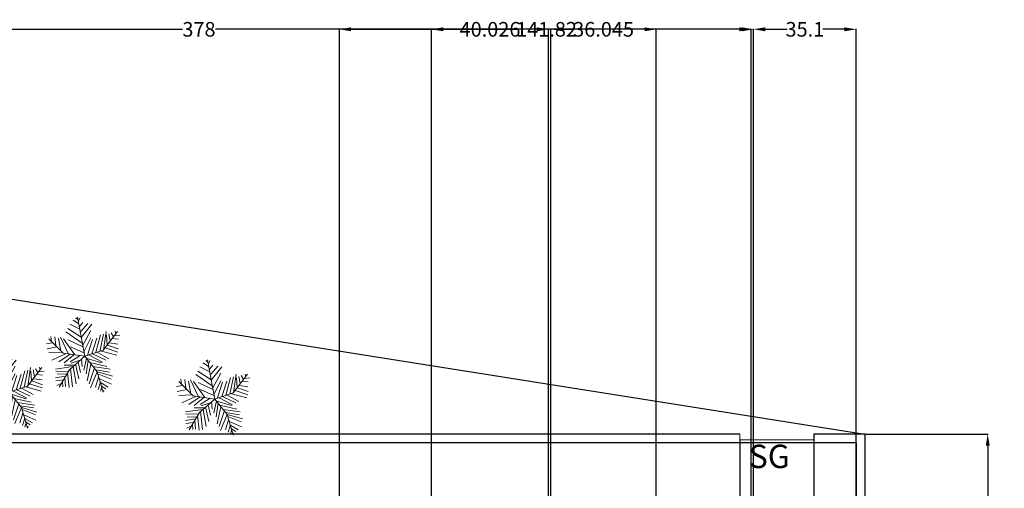
# Model space of a CAD drawing. Units: inches. Extents: x 460 to 1030, y -658 to 271.
# Tile 10 of 10: x 690 to 1028, y 111 to 271. Entities that reach past the tile are written whole.
import ezdxf

# ---------------------------------------------------------------- set-up
doc = ezdxf.new("R2010")
doc.units = ezdxf.units.IN
doc.header["$MEASUREMENT"] = 0
for name, color, linetype, lineweight in [('A-ANNO-DIMS', 2, 'Continuous', 18), ('A-ANNO-TEXT', 7, 'Continuous', 18), ('C-PROP', 7, 'Continuous', 25), ('C-SITE-GATE', 3, 'Continuous', 18), ('L-PLNT', 94, 'Continuous', 13)]:
    doc.layers.add(name, color=color, linetype=linetype, lineweight=lineweight)
doc.styles.get("Standard").update_dxf_attribs({"font": 'arial.ttf'})
doc.dimstyles.get("Standard").update_dxf_attribs({"dimtxt": 5, "dimasz": 4, "dimexe": 0.18, "dimexo": 0.0625, "dimgap": 0.09, "dimtad": 0, "dimtih": 1, "dimtoh": 1, "dimdec": 1, "dimzin": 0, "dimdsep": 46, "dimlunit": 4, "dimtxsty": 'Standard', "dimcen": 0.09, "dimadec": 0, "dimazin": 0, "dimtfac": 1, "dimtdec": 1, "dimtofl": 0, "dimtmove": 0, "dimatfit": 3, "dimfxl": 1, "dimtolj": 1, "dimtzin": 0, "dimarcsym": 0})

# ---------------------------------------------------------------- blocks, each defined once
blk = doc.blocks.new('*U11')
for p, q in [((-185.1152, 1008.5578), (-553.1612, 1185.4942)), ((-221.9198, 1197.3052), (-433.5526, 1338.8594)), ((-258.7244, 1362.456), (-332.3336, 1421.4348)), ((0, 0), (-266.7, 1447.8)), ((-231.1146, 1315.2628), (-166.7002, 1421.4348)), ((-194.31, 1102.9442), (-65.4812, 1256.284)), ((-148.3106, 914.1968), (118.5418, 1220.9018)), ((-129.8956, 701.8528), (265.7602, 1185.4942)), ((-1234.059, 536.7274), (-1252.4486, 737.2604)), ((-93.091, 489.5342), (-700.3796, 902.3858)), ((-129.8956, 713.6638), (-626.7704, 1032.1544)), ((-74.7014, 418.7444), (219.7608, 961.39)), ((412.9786, 147.447), (587.8068, 796.2392)), ((560.197, 182.8292), (698.2206, 819.8358)), ((685.8, 228.6), (1219.2, 914.4)), ((689.0258, 230.0224), (790.2448, 914.1968)), ((808.6344, 784.4282), (827.0494, 418.7444)), ((891.4384, 831.6214), (946.658, 572.1096)), ((983.4626, 867.0036), (1066.2666, 725.4494)), ((1112.2914, 760.8316), (1296.3144, 784.4282)), ((1121.4862, 925.9824), (1149.0706, 831.6214)), ((-1206.4492, 501.3198), (-1418.082, 465.9376)), ((-800.1, 114.3), (-1333.5, 647.7)), ((-1105.2302, 725.4494), (-1077.6458, 395.1732)), ((-976.4268, 666.4706), (-884.4026, 194.6402)), ((-902.8176, 713.6638), (-617.5756, 100.2538)), ((-369.1382, 53.086), (-783.1836, 642.874)), ((-617.5756, 607.4918), (-74.7014, 347.98)), ((-28.6766, 171.0436), (228.9556, 678.2816)), ((100.1268, 41.275), (284.1498, 619.2774)), ((256.5654, 88.4682), (449.7832, 666.4706)), ((845.439, 418.7444), (1241.0948, 277.1902)), ((919.0482, 501.3198), (1222.6798, 454.152)), ((1029.462, 654.685), (1241.0948, 631.0884)), ((-1031.621, 347.98), (-1399.667, 277.1902)), ((-847.598, 159.2326), (-1326.0578, 135.636)), ((-718.7946, 88.4682), (-1215.644, -147.447)), ((-543.9664, 76.6572), (-967.2066, -206.4512)), ((0, 0), (-800.1, 114.3)), ((-405.9428, 53.086), (-764.794, -241.8334)), ((0, 0), (-571.5, -495.3)), ((-166.7002, 29.4894), (-543.9664, -206.4512)), ((-525.5514, 347.98), (-28.6766, 123.8504)), ((0, 0), (685.8, 228.6)), ((0, 0), (457.2, -571.5)), ((164.5412, 41.275), (661.416, -218.2368)), ((284.1498, 88.4682), (781.0246, -147.447)), ((458.978, 147.447), (891.4384, -88.4682)), ((615.4166, 194.6402), (1185.8752, 41.275)), ((753.4148, 312.5978), (1222.6798, 159.2326)), ((-387.5278, -324.4088), (-764.794, -324.4088)), ((-166.7002, -147.447), (-507.1618, -253.619)), ((-341.5284, -289.0012), (-221.9198, -831.6214)), ((-240.3094, -218.2368), (-157.5054, -595.7062)), ((-120.7008, -88.4682), (-93.091, -371.5766)), ((63.3222, -76.6826), (-37.8714, -513.1308)), ((44.9326, -64.897), (615.4166, -241.8334)), ((127.7366, -159.258), (54.1274, -654.685)), ((228.9556, -289.0012), (90.932, -914.1968)), ((192.151, -230.0224), (817.8292, -371.5766)), ((-442.7474, -383.3876), (-1086.8406, -477.7486)), ((-617.5756, -548.5384), (-1077.6458, -560.324)), ((-681.9646, -666.496), (-1022.4262, -654.685)), ((-571.5, -495.3), (-952.5, -1143)), ((-635.9652, -607.5172), (-580.771, -1150.1374)), ((-525.5514, -465.963), (-451.9422, -1126.5408)), ((-433.5526, -383.3876), (-323.1134, -1020.3688)), ((357.759, -430.5554), (164.5412, -1020.3688)), ((458.978, -572.1096), (210.5406, -1161.923)), ((311.7596, -383.3876), (937.4378, -477.7486)), ((412.9786, -501.3452), (919.0482, -583.9206)), ((457.2, -571.5), (685.8, -1333.5)), ((468.1982, -572.1096), (1029.462, -737.2604)), ((486.5878, -642.8994), (983.4626, -843.4324)), ((-718.7946, -737.2604), (-1086.8406, -796.2392)), ((-783.1836, -867.029), (-1077.6458, -902.4112)), ((-875.2078, -1008.5832), (-1040.8412, -1079.3476)), ((-829.2084, -937.7934), (-810.7934, -1126.5408)), ((-737.1842, -784.4536), (-709.5744, -1114.7298)), ((514.1976, -772.6426), (403.7838, -1138.3264)), ((578.612, -961.39), (495.7826, -1232.7128)), ((541.8074, -831.6214), (992.6574, -1032.1544)), ((578.612, -973.1756), (873.0488, -1138.3264)), ((624.6114, -1161.923), (587.8068, -1291.6916)), ((624.6114, -1102.9442), (781.0246, -1209.1162)), ((679.8056, -1268.095), (716.6102, -1291.6916))]:
    blk.add_line(p, q)
blk = doc.blocks.new('*D41')
at = {"layer": 'A-ANNO-DIMS', "color": 0, "lineweight": -2, "transparency": 16777216}
for p, q in [((979.86, 129.27), (1022.03, 129.27)), ((1021.85, 125.27), (1021.85, -76.63)), ((1021.85, -283.73), (1021.85, -81.83)), ((940.86, -287.73), (1022.03, -287.73))]:
    blk.add_line(p, q, dxfattribs=at)
at = {"layer": 'A-ANNO-DIMS', "color": 0, "transparency": 16777216}
for points in [[(1021.18, 125.27), (1022.51, 125.27), (1021.85, 129.27)], [(1021.18, -283.73), (1022.51, -283.73), (1021.85, -287.73)]]:
    blk.add_solid(points, dxfattribs=at)
at = {"layer": 'Defpoints', "color": 0, "transparency": 16777216}
for p in [(979.8, 129.27), (1021.85, 129.27), (940.8, -287.73)]:
    blk.add_point(p, dxfattribs=at)
at = {"layer": 'A-ANNO-DIMS', "color": 0, "transparency": 16777216, "insert": (1021.85, -79.23), "char_height": 5, "attachment_point": 5}
blk.add_mtext('\\A1;417', dxfattribs=at)
blk = doc.blocks.new('*D43')
at = {"layer": 'A-ANNO-DIMS', "color": 0, "lineweight": -2, "transparency": 16777216}
for p, q in [((562.8, 90.34), (562.8, 267.89)), ((566.8, 267.71), (746.18, 267.71)), ((936.8, 267.71), (757.41, 267.71)), ((940.8, 90.34), (940.8, 267.89))]:
    blk.add_line(p, q, dxfattribs=at)
at = {"layer": 'A-ANNO-DIMS', "color": 0, "transparency": 16777216}
for points in [[(566.8, 268.38), (566.8, 267.04), (562.8, 267.71)], [(936.8, 268.38), (936.8, 267.04), (940.8, 267.71)]]:
    blk.add_solid(points, dxfattribs=at)
at = {"layer": 'Defpoints', "color": 0, "transparency": 16777216}
for p in [(940.8, 267.71), (562.8, 90.27), (940.8, 90.27)]:
    blk.add_point(p, dxfattribs=at)
at = {"layer": 'A-ANNO-DIMS', "color": 0, "transparency": 16777216, "insert": (751.8, 267.71), "char_height": 5, "attachment_point": 5}
blk.add_mtext('\\A1;378', dxfattribs=at)
blk = doc.blocks.new('*D45')
at = {"layer": 'A-ANNO-DIMS', "color": 0, "lineweight": -2, "transparency": 16777216}
for p, q in [((976.8, 126.21), (976.8, -654.61)), ((940.8, 90.21), (940.8, -654.61)), ((944.8, -654.43), (955.13, -654.43)), ((972.8, -654.43), (962.46, -654.43))]:
    blk.add_line(p, q, dxfattribs=at)
at = {"layer": 'A-ANNO-DIMS', "color": 0, "transparency": 16777216}
for points in [[(944.8, -653.77), (944.8, -655.1), (940.8, -654.43)], [(972.8, -653.77), (972.8, -655.1), (976.8, -654.43)]]:
    blk.add_solid(points, dxfattribs=at)
at = {"layer": 'Defpoints', "color": 0, "transparency": 16777216}
for p in [(976.8, 126.27), (940.8, 90.27), (976.8, -654.43)]:
    blk.add_point(p, dxfattribs=at)
at = {"layer": 'A-ANNO-DIMS', "color": 0, "transparency": 16777216, "insert": (958.8, -654.43), "char_height": 5, "attachment_point": 5}
blk.add_mtext('\\A1;36', dxfattribs=at)
blk = doc.blocks.new('*D46')
at = {"layer": 'A-ANNO-DIMS', "color": 0, "lineweight": -2, "transparency": 16777216}
for p, q in [((936.98, 127.21), (936.98, -654.61)), ((962.32, 127.21), (962.32, -654.61)), ((932.98, -654.43), (928.98, -654.43)), ((966.32, -654.43), (970.32, -654.43))]:
    blk.add_line(p, q, dxfattribs=at)
at = {"layer": 'A-ANNO-DIMS', "color": 0, "transparency": 16777216}
for points in [[(932.98, -653.77), (932.98, -655.1), (936.98, -654.43)], [(966.32, -653.77), (966.32, -655.1), (962.32, -654.43)]]:
    blk.add_solid(points, dxfattribs=at)
at = {"layer": 'Defpoints', "color": 0, "transparency": 16777216}
for p in [(936.98, 127.27), (962.32, 127.27), (962.32, -654.43)]:
    blk.add_point(p, dxfattribs=at)
at = {"layer": 'A-ANNO-DIMS', "color": 0, "transparency": 16777216, "insert": (949.65, -654.43), "char_height": 5, "attachment_point": 5}
blk.add_mtext('\\A1;25.346', dxfattribs=at)
blk = doc.blocks.new('*D47')
at = {"layer": 'A-ANNO-DIMS', "color": 0, "lineweight": -2, "transparency": 16777216}
for p, q in [((962.32, 129.21), (962.32, -654.61)), ((979.8, 129.21), (979.8, -654.61)), ((966.32, -654.43), (975.8, -654.43)), ((979.8, -654.43), (983.8, -654.43))]:
    blk.add_line(p, q, dxfattribs=at)
at = {"layer": 'A-ANNO-DIMS', "color": 0, "transparency": 16777216}
for points in [[(966.32, -653.77), (966.32, -655.1), (962.32, -654.43)], [(975.8, -653.77), (975.8, -655.1), (979.8, -654.43)]]:
    blk.add_solid(points, dxfattribs=at)
at = {"layer": 'Defpoints', "color": 0, "transparency": 16777216}
for p in [(962.32, 129.27), (979.8, 129.27), (979.8, -654.43)]:
    blk.add_point(p, dxfattribs=at)
at = {"layer": 'A-ANNO-DIMS', "color": 0, "transparency": 16777216, "insert": (994.02, -654.43), "char_height": 5, "attachment_point": 5}
blk.add_mtext('\\A1;17.474', dxfattribs=at)
blk = doc.blocks.new('*D48')
at = {"layer": 'A-ANNO-DIMS', "color": 0, "lineweight": -2, "transparency": 16777216}
for p, q in [((799.88, -611.66), (799.88, 267.89)), ((803.88, 267.71), (860.58, 267.71)), ((937.7, 267.71), (881, 267.71)), ((941.7, -611.66), (941.7, 267.89))]:
    blk.add_line(p, q, dxfattribs=at)
at = {"layer": 'A-ANNO-DIMS', "color": 0, "transparency": 16777216}
for points in [[(803.88, 268.38), (803.88, 267.04), (799.88, 267.71)], [(937.7, 268.38), (937.7, 267.04), (941.7, 267.71)]]:
    blk.add_solid(points, dxfattribs=at)
at = {"layer": 'Defpoints', "color": 0, "transparency": 16777216}
for p in [(941.7, 267.71), (799.88, -611.73), (941.7, -611.73)]:
    blk.add_point(p, dxfattribs=at)
at = {"layer": 'A-ANNO-DIMS', "color": 0, "transparency": 16777216, "insert": (870.79, 267.71), "char_height": 5, "attachment_point": 5}
blk.add_mtext('\\A1;141.82', dxfattribs=at)
blk = doc.blocks.new('*D49')
at = {"layer": 'A-ANNO-DIMS', "color": 0, "lineweight": -2, "transparency": 16777216}
for p, q in [((941.7, -608.66), (941.7, 267.89)), ((945.7, 267.71), (953.15, 267.71)), ((972.8, 267.71), (965.35, 267.71)), ((976.8, -608.66), (976.8, 267.89))]:
    blk.add_line(p, q, dxfattribs=at)
at = {"layer": 'A-ANNO-DIMS', "color": 0, "transparency": 16777216}
for points in [[(945.7, 268.38), (945.7, 267.04), (941.7, 267.71)], [(972.8, 268.38), (972.8, 267.04), (976.8, 267.71)]]:
    blk.add_solid(points, dxfattribs=at)
at = {"layer": 'Defpoints', "color": 0, "transparency": 16777216}
for p in [(976.8, 267.71), (941.7, -608.73), (976.8, -608.73)]:
    blk.add_point(p, dxfattribs=at)
at = {"layer": 'A-ANNO-DIMS', "color": 0, "transparency": 16777216, "insert": (959.25, 267.71), "char_height": 5, "attachment_point": 5}
blk.add_mtext('\\A1;35.1', dxfattribs=at)
blk = doc.blocks.new('*D52')
at = {"layer": 'A-ANNO-DIMS', "color": 0, "lineweight": -2, "transparency": 16777216}
for p, q in [((872.3, -281.66), (872.3, 267.89)), ((876.3, 267.71), (879.84, 267.71)), ((904.35, 267.71), (900.81, 267.71)), ((908.35, -281.66), (908.35, 267.89))]:
    blk.add_line(p, q, dxfattribs=at)
at = {"layer": 'A-ANNO-DIMS', "color": 0, "transparency": 16777216}
for points in [[(876.3, 268.38), (876.3, 267.04), (872.3, 267.71)], [(904.35, 268.38), (904.35, 267.04), (908.35, 267.71)]]:
    blk.add_solid(points, dxfattribs=at)
at = {"layer": 'Defpoints', "color": 0, "transparency": 16777216}
for p in [(908.35, 267.71), (872.3, -281.73), (908.35, -281.73)]:
    blk.add_point(p, dxfattribs=at)
at = {"layer": 'A-ANNO-DIMS', "color": 0, "transparency": 16777216, "insert": (890.32, 267.71), "char_height": 5, "attachment_point": 5}
blk.add_mtext('\\A1;36.045', dxfattribs=at)
blk = doc.blocks.new('*D71')
at = {"layer": 'A-ANNO-DIMS', "color": 0, "lineweight": -2, "transparency": 16777216}
for p, q in [((831.43, -281.66), (831.43, 267.89)), ((835.43, 267.71), (840.88, 267.71)), ((867.46, 267.71), (862.01, 267.71)), ((871.46, -281.66), (871.46, 267.89))]:
    blk.add_line(p, q, dxfattribs=at)
at = {"layer": 'A-ANNO-DIMS', "color": 0, "transparency": 16777216}
for points in [[(835.43, 268.38), (835.43, 267.04), (831.43, 267.71)], [(867.46, 268.38), (867.46, 267.04), (871.46, 267.71)]]:
    blk.add_solid(points, dxfattribs=at)
at = {"layer": 'Defpoints', "color": 0, "transparency": 16777216}
for p in [(871.46, 267.71), (831.43, -281.73), (871.46, -281.73)]:
    blk.add_point(p, dxfattribs=at)
at = {"layer": 'A-ANNO-DIMS', "color": 0, "transparency": 16777216, "insert": (851.44, 267.71), "char_height": 5, "attachment_point": 5}
blk.add_mtext('\\A1;40.026', dxfattribs=at)

msp = doc.modelspace()

# ---------------------------------------------------------------- linework, layer by layer
at = {"layer": 'C-PROP'}
for p, q in [((523.7961, 201.2738), (979.7961, 129.2738)), ((936.9757, 129.2738), (523.7961, 129.2738)), ((979.7961, 129.2738), (962.3217, 129.2738)), ((979.7961, 129.2738), (979.7961, -524.7262)), ((976.7961, 126.2738), (526.7961, 126.2738)), ((976.7961, 126.2738), (976.7961, -466.833))]:
    msp.add_line(p, q, dxfattribs=at)
at = {"layer": 'C-SITE-GATE'}
for p, q in [((936.9757, 126.2738), (936.9757, 129.2738)), ((962.3217, 126.2738), (962.3217, 129.2738)), ((962.3217, 127.2738), (936.9757, 127.2738)), ((962.3217, 126.2738), (936.9757, 126.2738))]:
    msp.add_line(p, q, dxfattribs=at)

# ---------------------------------------------------------------- block references
at = {"layer": 'L-PLNT', "xscale": 0.0092368434635362, "yscale": 0.0092368434635362, "zscale": 0.0092368434635362}
for p in [(712.6975, 155.8493), (686.7899, 143.5676), (757.2055, 141.244)]:
    msp.add_blockref('*U11', p, dxfattribs=at)

# ---------------------------------------------------------------- texts
at = {"layer": 'A-ANNO-TEXT'}
msp.add_text('SG', height=8, dxfattribs=at).set_placement((940.0514, 117.6177))

# ---------------------------------------------------------------- dimensions: what is measured, and where the dimension line sits
at = {"layer": 'A-ANNO-DIMS'}
for base, p1, p2, override, picture, middle in [((940.7961, 267.7108), (562.7961, 90.2738), (940.7961, 90.2738), {"dimdec": 0, "dimlfac": 1, "dimrnd": 0, "dimzin": 0, "dimdsep": 46, "dimlunit": 2}, '*D43', (751.7961, 267.7108)), ((941.6978, 267.7108), (799.8801, -611.7262), (941.6978, -611.7262), {"dimdec": 2, "dimlfac": 1, "dimrnd": 0, "dimzin": 0, "dimdsep": 46, "dimlunit": 2}, '*D48', (870.7889, 267.7108)), ((871.4559, 267.7108), (831.4302, -281.7262), (871.4559, -281.7262), {"dimdec": 3, "dimlfac": 1, "dimrnd": 0, "dimzin": 0, "dimdsep": 46, "dimlunit": 2}, '*D71', (851.443, 267.7108)), ((908.3452, 267.7108), (872.2999, -281.7262), (908.3452, -281.7262), {"dimdec": 3, "dimlfac": 1, "dimrnd": 0, "dimzin": 0, "dimdsep": 46, "dimlunit": 2}, '*D52', (890.3226, 267.7108)), ((976.7961, 267.7108), (941.6978, -608.7262), (976.7961, -608.7262), {"dimdec": 1, "dimlfac": 1, "dimrnd": 0, "dimzin": 0, "dimdsep": 46, "dimlunit": 2}, '*D49', (959.247, 267.7108)), ((979.7961, -654.4339), (962.3217, 129.2738), (979.7961, 129.2738), {"dimdec": 3, "dimlfac": 1, "dimrnd": 0, "dimzin": 0, "dimdsep": 46, "dimlunit": 2}, '*D47', (994.0191, -654.4339)), ((962.3217, -654.4339), (936.9757, 127.2738), (962.3217, 127.2738), {"dimdec": 3, "dimlfac": 1, "dimrnd": 0, "dimzin": 0, "dimdsep": 46, "dimlunit": 2}, '*D46', (949.6487, -654.4339)), ((976.7961, -654.4339), (940.7961, 90.2738), (976.7961, 126.2738), {"dimdec": 0, "dimlfac": 1, "dimrnd": 0, "dimzin": 0, "dimdsep": 46, "dimlunit": 2}, '*D45', (958.7961, -654.4339))]:
    dim = msp.add_linear_dim(base=base, p1=p1, p2=p2, dimstyle='Standard', override=override, dxfattribs=at)
    dim.commit()
    dim.dimension.update_dxf_attribs({"geometry": picture, "text_midpoint": middle})
dim = msp.add_linear_dim(base=(1021.8461, 129.2738), p1=(940.7961, -287.7262), p2=(979.7961, 129.2738), angle=90, dimstyle='Standard', override={"dimdec": 0, "dimlfac": 1, "dimrnd": 0, "dimzin": 0, "dimdsep": 46, "dimlunit": 2}, dxfattribs=at)
dim.commit()
dim.dimension.update_dxf_attribs({"geometry": '*D41', "text_midpoint": (1021.8461, -79.2262)})

doc.saveas('drawing.dxf')
